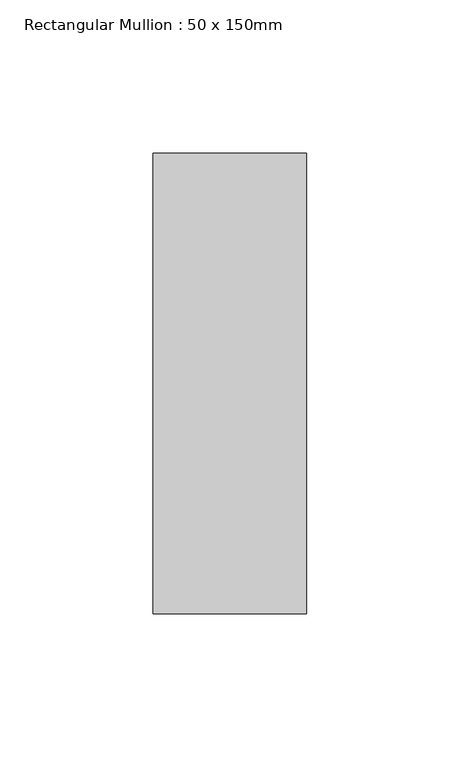
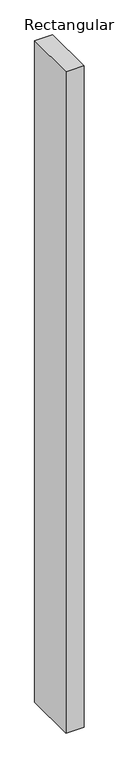
"""IFC4 building model written with IfcOpenShell, lengths in millimetres: member geometry, Rectangular Mullion : 50 x 150mm."""

from ifc_helpers import new_model, si_unit, frame, origin, place, context, project, spatial, polyline, outline, extrude, source, transform, mapped, element, save


def rectangular_mullion_50_x_150mm_6afb4452(model_context):
    return source(origin(), model_context, "Body", "SweptSolid", [
        extrude(outline(polyline([(0.0, 75.0), (0.0, -75.0), (-50.0, -75.0), (-50.0, 75.0), (0.0, 75.0)])), frame((0.0, 0.0, -1940.4113705), z_axis=(0.0, 0.0, 1.0), x_axis=(1.0, 0.0, 0.0)), (0.0, 0.0, 1.0), 1940.4113705),
    ])


if __name__ == "__main__":
    model = new_model("IFC4")
    model_context = context("Model", 3, world=origin())
    ifc_project = project(units=[si_unit("LENGTHUNIT", "METRE", prefix="MILLI")], contexts=[model_context])
    site = spatial("IfcSite", under=ifc_project)
    building = spatial("IfcBuilding", under=site)
    placement = place(None, origin())
    rectangular_mullion_50_x_150mm_shape = rectangular_mullion_50_x_150mm_6afb4452(model_context)
    element("IfcMember", 1, ObjectType="Rectangular Mullion : 50 x 150mm", at=placement, inside=building, context=model_context, shape_type="MappedRepresentation", body=[
        mapped(rectangular_mullion_50_x_150mm_shape, transform((0.0, 0.0, 0.0), x_axis=(1.0, 0.0, 0.0), y_axis=(0.0, 1.0, 0.0), z_axis=(0.0, 0.0, 1.0))),
    ])
    save(model, "model.ifc")

# Revit data of these elements
# Type "Rectangular Mullion : 50 x 150mm"
#   built-in parameter 1007304 = 0.492126 (stored number, unit not read)
#   built-in parameter 1007301 = 0.082021 (stored number, unit not read)
#   built-in parameter 1007300 = 0.082021 (stored number, unit not read)
# Element 1 (IfcMember, "Rectangular Mullion : 50 x 150mm")
#   Materials on its faces: "Aluminium"
# Materials
#   "Aluminium": class "Metal", colour RGB 247 247 247, transparency 0, Description = "Aluminium 6061", Cost = 0
